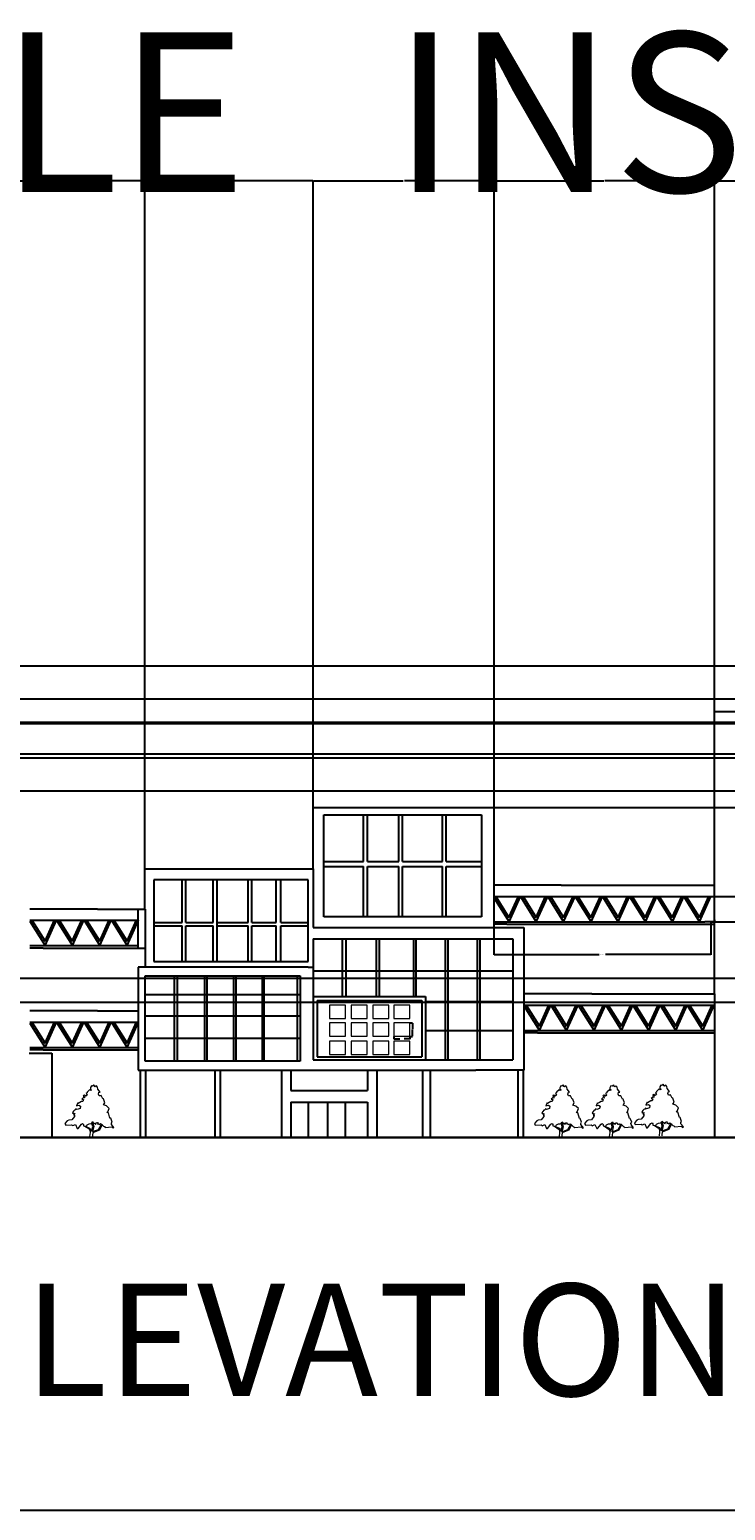
# Model space of a CAD drawing. Units: inches. Extents: x -2248 to 2617, y -128 to 922.
# Tile 3 of 7: x -646 to -152, y -128 to 922. Entities that reach past the tile are written whole.
import ezdxf

# ---------------------------------------------------------------- set-up
doc = ezdxf.new("R2010")
doc.units = ezdxf.units.IN
doc.header["$MEASUREMENT"] = 0
for name, color, linetype, lineweight in [('A-ANNO-DIMS', 2, 'Continuous', 18), ('A-ANNO-TEXT', 7, 'Continuous', 25), ('A-ELEV', 7, 'Continuous', 25), ('A-GLAZ', 4, 'Continuous', 18), ('L-PLNT', 3, 'Continuous', 18)]:
    doc.layers.add(name, color=color, linetype=linetype, lineweight=lineweight)
doc.styles.get("Standard").update_dxf_attribs({"font": 'arial.ttf'})
doc.dimstyles.get("Standard").update_dxf_attribs({"dimtxt": 0.18, "dimasz": 0.18, "dimexe": 0.18, "dimexo": 0.0625, "dimgap": 0.09, "dimtad": 0, "dimtih": 1, "dimtoh": 1, "dimdec": 4, "dimzin": 0, "dimdsep": 46, "dimtxsty": 'Standard', "dimcen": 0.09, "dimadec": 0, "dimazin": 0, "dimtfac": 1, "dimtdec": 4, "dimtofl": 0, "dimtmove": 0, "dimatfit": 3, "dimfxl": 1, "dimtolj": 1, "dimtzin": 0, "dimarcsym": 0})

# ---------------------------------------------------------------- blocks, each defined once
blk = doc.blocks.new('*U2')
for points in [[(22.0124, 137.721), (18.5475, 141.5624), (15.5282, 138.2446), (13.8028, 139.3505), (13.3714, 142.1153), (11.2148, 143.2214), (8.1954, 140.4564), (4.7447, 141.0094), (2.1567, 136.0326), (2.1567, 131.6088), (5.6074, 129.9499), (3.0193, 128.2909), (0.4313, 130.5029), (-6.9015, 123.3141), (-6.9015, 121.6552), (-9.9208, 119.9963), (-9.0581, 118.3373), (-6.9015, 115.0195), (-10.7835, 112.2546), (-14.6656, 115.0195), (-16.8222, 114.4665), (-17.6849, 112.2546), (-14.6656, 111.7016), (-14.2342, 107.2778), (-17.6065, 107.8307), (-21.5669, 103.9599), (-17.2536, 103.4069), (-18.9789, 97.8771), (-22.8609, 97.3241), (-27.1743, 94.5593), (-32.3504, 91.7944), (-32.7817, 94.0063), (-36.6638, 85.7116), (-29.7624, 87.3705), (-25.449, 84.6056), (-26.743, 77.9699), (-34.507, 75.205), (-37.9578, 77.4169), (-39.2518, 74.099), (-42.2711, 73.5461), (-44.8592, 70.2282), (-47.8786, 66.3574), (-43.9965, 63.0395), (-41.4085, 64.6985), (-44.3346, 59.8898), (-42.2089, 60.1377), (-42.5159, 55.7849), (-49.6039, 46.4502), (-58.2307, 45.8972), (-62.1127, 43.6853), (-68.5828, 36.4966), (-65.9947, 32.0727), (-50.0352, 32.6257), (-47.0159, 30.4138), (-39.6831, 33.7317), (-34.507, 22.6721), (-32.3504, 22.6721), (-22.4296, 34.8376), (-19.4102, 36.4966), (-17.2536, 33.7317), (-17.2536, 29.8608), (-13.8028, 28.7549), (-9.0581, 28.7549), (-7.3328, 32.6257), (-1.7254, 35.3906), (3.8821, 35.9436), (6.4701, 38.1555), (6.9014, 38.7085), (8.1954, 41.4734), (9.9208, 40.3674), (11.2148, 35.9436), (14.2341, 37.6025), (15.0968, 36.4966), (15.9595, 33.7317), (18.9789, 38.7085), (21.9982, 38.7085), (23.2922, 36.4966), (21.9982, 34.2847), (25.4489, 35.3906), (26.743, 33.7317), (29.7623, 35.9436), (32.7817, 34.8376), (38.8204, 28.7549), (41.4084, 27.6489), (43.5651, 25.437), (61.6813, 27.0959), (65.132, 23.7781), (67.7201, 24.884), (60.8186, 33.7317), (60.3873, 37.0495), (62.544, 40.3674), (58.662, 50.874), (56.5053, 50.874), (52.1919, 66.3574), (47.8785, 66.9103), (50.4665, 69.1222), (53.9172, 77.9699), (47.0158, 85.1586), (38.3891, 87.9235), (42.2711, 94.0063)], [(42.2711, 94.0063), (38.8204, 104.5129), (36.6637, 104.5129), (32.3503, 113.9135), (29.7623, 113.3605), (26.743, 113.3605), (24.5862, 117.7844), (25.8802, 123.8671), (29.331, 123.8671), (22.8609, 131.6088), (21.9982, 137.6916)], [(-12.9401, 28.7549), (-2.588, 22.1191), (0.8626, 17.6953), (1.7253, 11.6125), (0, 0)], [(-9.9208, 28.2019), (0, 23.2251), (3.4507, 19.9072), (4.7447, 15.4834), (8.6267, 27.0959), (6.4701, 37.6025)], [(34.5071, 33.1787), (27.1743, 18.2483), (9.0581, 10.5066), (7.7641, 3.8708), (8.1954, 0)], [(8.1954, 40.3674), (11.2148, 27.6489), (8.1954, 13.8245), (24.5862, 19.9072), (32.7817, 34.2847)]]:
    blk.add_lwpolyline(points)
blk = doc.blocks.new('TRUSS-BRIDGE-SEG')
for p, q in [((0, 17.2), (10.8, 0)), ((10.8, 0), (18.9, 17.9)), ((18.8, 17.9), (30.1, 0)), ((30.1, 0), (38.2, 17.9)), ((38.3, 17.9), (49.5, 0)), ((49.5, 0), (57.6, 17.9)), ((57.7, 17.9), (69, 0)), ((69, 0), (77.1, 17.9)), ((77, 17.9), (88.2, 0)), ((88.2, 0), (96.3, 17.9)), ((96.3, 17.9), (107.5, 0)), ((107.5, 0), (115.6, 17.9)), ((115.5, 17.9), (126.7, 0)), ((126.7, 0), (134.8, 17.9)), ((134.7, 17.9), (145.9, 0)), ((145.9, 0), (154, 17.9))]:
    blk.add_line(p, q)
blk = doc.blocks.new('WIN-SMALL')
for p, q in [((0, 9.6), (0, 0)), ((11.4, 9.6), (0, 9.6)), ((0, 0), (11.4, 0)), ((11.4, 0), (11.4, 9.6))]:
    blk.add_line(p, q)
blk = doc.blocks.new('*D8')
at = {"layer": 'A-ANNO-DIMS', "color": 0, "lineweight": -2, "transparency": 16777216}
for p, q in [((-387.2, 208.1), (-387.2, 206.2)), ((-387, 206.4), (-383.1, 206.4)), ((-376, 206.4), (-380, 206.4)), ((-375.8, 208.1), (-375.8, 206.2))]:
    blk.add_line(p, q, dxfattribs=at)
at = {"layer": 'A-ANNO-DIMS', "color": 0, "transparency": 16777216}
for points in [[(-387, 206.5), (-387, 206.4), (-387.2, 206.4)], [(-376, 206.5), (-376, 206.4), (-375.8, 206.4)]]:
    blk.add_solid(points, dxfattribs=at)
at = {"layer": 'Defpoints', "color": 0, "transparency": 16777216}
for p in [(-387.2, 208.1), (-375.8, 208.1), (-375.8, 206.4)]:
    blk.add_point(p, dxfattribs=at)
at = {"layer": 'A-ANNO-DIMS', "color": 0, "transparency": 16777216, "insert": (-381.5, 206.4), "char_height": 0.18, "attachment_point": 5}
blk.add_mtext('\\A1;SMALL WINDOW 11 TYP.', dxfattribs=at)
blk = doc.blocks.new('*D9')
at = {"layer": 'A-ANNO-DIMS', "color": 0, "lineweight": -2, "transparency": 16777216}
for p, q in [((-375.8, 217.7), (-374, 217.7)), ((-374.1, 217.5), (-374.1, 213.1)), ((-374.1, 208.3), (-374.1, 212.7)), ((-375.8, 208.1), (-374, 208.1))]:
    blk.add_line(p, q, dxfattribs=at)
at = {"layer": 'A-ANNO-DIMS', "color": 0, "transparency": 16777216}
for points in [[(-374.2, 217.5), (-374.1, 217.5), (-374.1, 217.7)], [(-374.2, 208.3), (-374.1, 208.3), (-374.1, 208.1)]]:
    blk.add_solid(points, dxfattribs=at)
at = {"layer": 'Defpoints', "color": 0, "transparency": 16777216}
for p in [(-375.8, 217.7), (-374.1, 217.7), (-375.8, 208.1)]:
    blk.add_point(p, dxfattribs=at)
at = {"layer": 'A-ANNO-DIMS', "color": 0, "transparency": 16777216, "insert": (-374.1, 212.9), "char_height": 0.18, "attachment_point": 5}
blk.add_mtext('\\A1;10 TYP.', dxfattribs=at)
blk = doc.blocks.new('*D14')
at = {"layer": 'A-ANNO-DIMS', "color": 0, "lineweight": -2, "transparency": 16777216}
for p, q in [((-316.3, 289.2), (-316.3, 266)), ((-162.4, 289.2), (-162.4, 266)), ((-316.1, 266.2), (-241.6, 266.2)), ((-162.5, 266.2), (-237.1, 266.2))]:
    blk.add_line(p, q, dxfattribs=at)
at = {"layer": 'A-ANNO-DIMS', "color": 0, "transparency": 16777216}
for points in [[(-316.1, 266.2), (-316.1, 266.2), (-316.3, 266.2)], [(-162.5, 266.2), (-162.5, 266.2), (-162.4, 266.2)]]:
    blk.add_solid(points, dxfattribs=at)
at = {"layer": 'Defpoints', "color": 0, "transparency": 16777216}
for p in [(-316.3, 289.3), (-162.4, 289.3), (-162.4, 266.2)]:
    blk.add_point(p, dxfattribs=at)
at = {"layer": 'A-ANNO-DIMS', "color": 0, "transparency": 16777216, "insert": (-239.3, 266.2), "char_height": 0.18, "attachment_point": 5}
blk.add_mtext('\\A1;TRUSS BRIDGE SEGMENT 154 TYP.', dxfattribs=at)
blk = doc.blocks.new('*D15')
at = {"layer": 'A-ANNO-DIMS', "color": 0, "lineweight": -2, "transparency": 16777216}
for p, q in [((-162.3, 307.2), (-139.1, 307.2)), ((-139.3, 307), (-139.3, 298.4)), ((-139.3, 289.5), (-139.3, 298.1)), ((-162.3, 289.3), (-139.1, 289.3))]:
    blk.add_line(p, q, dxfattribs=at)
at = {"layer": 'A-ANNO-DIMS', "color": 0, "transparency": 16777216}
for points in [[(-139.3, 307), (-139.2, 307), (-139.3, 307.2)], [(-139.3, 289.5), (-139.2, 289.5), (-139.3, 289.3)]]:
    blk.add_solid(points, dxfattribs=at)
at = {"layer": 'Defpoints', "color": 0, "transparency": 16777216}
for p in [(-162.4, 307.2), (-139.3, 307.2), (-162.4, 289.3)]:
    blk.add_point(p, dxfattribs=at)
at = {"layer": 'A-ANNO-DIMS', "color": 0, "transparency": 16777216, "insert": (-139.3, 298.2), "char_height": 0.18, "attachment_point": 5}
blk.add_mtext('\\A1;18 TYP.', dxfattribs=at)
blk = doc.blocks.new('*D20')
at = {"layer": 'A-ANNO-DIMS', "color": 0, "lineweight": -2, "transparency": 16777216}
for p, q in [((-1595.3, 429.9), (2616.5, 429.9)), ((2616.3, 429.7), (2616.3, 417.9)), ((2616.3, 405.8), (2616.3, 417.5)), ((-1653.9, 405.6), (2616.5, 405.6))]:
    blk.add_line(p, q, dxfattribs=at)
at = {"layer": 'A-ANNO-DIMS', "color": 0, "transparency": 16777216}
for points in [[(2616.2, 429.7), (2616.3, 429.7), (2616.3, 429.9)], [(2616.2, 405.8), (2616.3, 405.8), (2616.3, 405.6)]]:
    blk.add_solid(points, dxfattribs=at)
at = {"layer": 'Defpoints', "color": 0, "transparency": 16777216}
for p in [(-1595.4, 429.9), (-1654, 405.6), (2616.3, 405.6)]:
    blk.add_point(p, dxfattribs=at)
at = {"layer": 'A-ANNO-DIMS', "color": 0, "transparency": 16777216, "insert": (2616.3, 417.7), "char_height": 0.18, "attachment_point": 5}
blk.add_mtext('\\A1;24.3', dxfattribs=at)
blk = doc.blocks.new('*D21')
at = {"layer": 'A-ANNO-DIMS', "color": 0, "lineweight": -2, "transparency": 16777216}
for p, q in [((-1125.3, 470.6), (2616.5, 470.6)), ((2616.3, 470.4), (2616.3, 451)), ((2616.3, 431.1), (2616.3, 450.6)), ((-1257.9, 430.9), (2616.5, 430.9))]:
    blk.add_line(p, q, dxfattribs=at)
at = {"layer": 'A-ANNO-DIMS', "color": 0, "transparency": 16777216}
for points in [[(2616.2, 470.4), (2616.3, 470.4), (2616.3, 470.6)], [(2616.2, 431.1), (2616.3, 431.1), (2616.3, 430.9)]]:
    blk.add_solid(points, dxfattribs=at)
at = {"layer": 'Defpoints', "color": 0, "transparency": 16777216}
for p in [(-1125.4, 470.6), (-1258, 430.9), (2616.3, 430.9)]:
    blk.add_point(p, dxfattribs=at)
at = {"layer": 'A-ANNO-DIMS', "color": 0, "transparency": 16777216, "insert": (2616.3, 450.8), "char_height": 0.18, "attachment_point": 5}
blk.add_mtext('\\A1;39.705', dxfattribs=at)
blk = doc.blocks.new('*D22')
at = {"layer": 'A-ANNO-DIMS', "color": 0, "lineweight": -2, "transparency": 16777216}
for p, q in [((-733.3, 408.4), (2616.5, 408.4)), ((2616.3, 408.2), (2616.3, 329.1)), ((2616.3, 249.6), (2616.3, 328.7)), ((-719.1, 249.4), (2616.5, 249.4))]:
    blk.add_line(p, q, dxfattribs=at)
at = {"layer": 'A-ANNO-DIMS', "color": 0, "transparency": 16777216}
for points in [[(2616.2, 408.2), (2616.3, 408.2), (2616.3, 408.4)], [(2616.2, 249.6), (2616.3, 249.6), (2616.3, 249.4)]]:
    blk.add_solid(points, dxfattribs=at)
at = {"layer": 'Defpoints', "color": 0, "transparency": 16777216}
for p in [(-733.4, 408.4), (-719.2, 249.4), (2616.3, 249.4)]:
    blk.add_point(p, dxfattribs=at)
at = {"layer": 'A-ANNO-DIMS', "color": 0, "transparency": 16777216, "insert": (2616.3, 328.9), "char_height": 0.18, "attachment_point": 5}
blk.add_mtext('\\A1;159.02', dxfattribs=at)
blk = doc.blocks.new('*D23')
at = {"layer": 'A-ANNO-DIMS', "color": 0, "lineweight": -2, "transparency": 16777216}
for p, q in [((-719.1, 249.4), (2616.5, 249.4)), ((2616.3, 249.2), (2616.3, 193.1)), ((2616.3, 136.6), (2616.3, 192.7)), ((-719.1, 136.5), (2616.5, 136.5))]:
    blk.add_line(p, q, dxfattribs=at)
at = {"layer": 'A-ANNO-DIMS', "color": 0, "transparency": 16777216}
for points in [[(2616.2, 249.2), (2616.3, 249.2), (2616.3, 249.4)], [(2616.2, 136.6), (2616.3, 136.6), (2616.3, 136.5)]]:
    blk.add_solid(points, dxfattribs=at)
at = {"layer": 'Defpoints', "color": 0, "transparency": 16777216}
for p in [(-719.2, 249.4), (-719.2, 136.5), (2616.3, 136.5)]:
    blk.add_point(p, dxfattribs=at)
at = {"layer": 'A-ANNO-DIMS', "color": 0, "transparency": 16777216, "insert": (2616.3, 192.9), "char_height": 0.18, "attachment_point": 5}
blk.add_mtext('\\A1;112.94', dxfattribs=at)
blk = doc.blocks.new('*D24')
at = {"layer": 'A-ANNO-DIMS', "color": 0, "lineweight": -2, "transparency": 16777216}
for p, q in [((-316.1, 370.3), (2616.5, 370.3)), ((2616.3, 370.1), (2616.3, 253.6)), ((2616.3, 136.6), (2616.3, 253.2)), ((-159.8, 136.5), (2616.5, 136.5))]:
    blk.add_line(p, q, dxfattribs=at)
at = {"layer": 'A-ANNO-DIMS', "color": 0, "transparency": 16777216}
for points in [[(2616.2, 370.1), (2616.3, 370.1), (2616.3, 370.3)], [(2616.2, 136.6), (2616.3, 136.6), (2616.3, 136.5)]]:
    blk.add_solid(points, dxfattribs=at)
at = {"layer": 'Defpoints', "color": 0, "transparency": 16777216}
for p in [(-316.2, 370.3), (-159.9, 136.5), (2616.3, 136.5)]:
    blk.add_point(p, dxfattribs=at)
at = {"layer": 'A-ANNO-DIMS', "color": 0, "transparency": 16777216, "insert": (2616.3, 253.4), "char_height": 0.18, "attachment_point": 5}
blk.add_mtext('\\A1;233.87', dxfattribs=at)
blk = doc.blocks.new('*D29')
at = {"layer": 'A-ANNO-DIMS', "color": 0, "lineweight": -2, "transparency": 16777216}
for p, q in [((358.9, 382), (-2247.7, 382)), ((-2247.5, 381.8), (-2247.5, 259.4)), ((-2247.5, 136.6), (-2247.5, 259)), ((392.6, 136.5), (-2247.7, 136.5))]:
    blk.add_line(p, q, dxfattribs=at)
at = {"layer": 'A-ANNO-DIMS', "color": 0, "transparency": 16777216}
for points in [[(-2247.5, 381.8), (-2247.5, 381.8), (-2247.5, 382)], [(-2247.5, 136.6), (-2247.5, 136.6), (-2247.5, 136.5)]]:
    blk.add_solid(points, dxfattribs=at)
at = {"layer": 'Defpoints', "color": 0, "transparency": 16777216}
for p in [(359, 382), (-2247.5, 136.5), (392.7, 136.5)]:
    blk.add_point(p, dxfattribs=at)
at = {"layer": 'A-ANNO-DIMS', "color": 0, "transparency": 16777216, "insert": (-2247.5, 259.2), "char_height": 0.18, "attachment_point": 5}
blk.add_mtext('\\A1;245.5', dxfattribs=at)
blk = doc.blocks.new('*D30')
at = {"layer": 'A-ANNO-DIMS', "color": 0, "lineweight": -2, "transparency": 16777216}
for p, q in [((201.8, 232.1), (-2247.7, 232.1)), ((-2247.5, 231.9), (-2247.5, 184.4)), ((-2247.5, 136.6), (-2247.5, 184.1)), ((210.7, 136.5), (-2247.7, 136.5))]:
    blk.add_line(p, q, dxfattribs=at)
at = {"layer": 'A-ANNO-DIMS', "color": 0, "transparency": 16777216}
for points in [[(-2247.5, 231.9), (-2247.5, 231.9), (-2247.5, 232.1)], [(-2247.5, 136.6), (-2247.5, 136.6), (-2247.5, 136.5)]]:
    blk.add_solid(points, dxfattribs=at)
at = {"layer": 'Defpoints', "color": 0, "transparency": 16777216}
for p in [(201.8, 232.1), (-2247.5, 136.5), (210.8, 136.5)]:
    blk.add_point(p, dxfattribs=at)
at = {"layer": 'A-ANNO-DIMS', "color": 0, "transparency": 16777216, "insert": (-2247.5, 184.3), "char_height": 0.18, "attachment_point": 5}
blk.add_mtext('\\A1;95.6', dxfattribs=at)
blk = doc.blocks.new('*D31')
at = {"layer": 'A-ANNO-DIMS', "color": 0, "lineweight": -2, "transparency": 16777216}
for p, q in [((934.8, 447.2), (-2247.7, 447.2)), ((-2247.5, 447), (-2247.5, 292)), ((-2247.5, 136.6), (-2247.5, 291.6)), ((820, 136.5), (-2247.7, 136.5))]:
    blk.add_line(p, q, dxfattribs=at)
at = {"layer": 'A-ANNO-DIMS', "color": 0, "transparency": 16777216}
for points in [[(-2247.5, 447), (-2247.5, 447), (-2247.5, 447.2)], [(-2247.5, 136.6), (-2247.5, 136.6), (-2247.5, 136.5)]]:
    blk.add_solid(points, dxfattribs=at)
at = {"layer": 'Defpoints', "color": 0, "transparency": 16777216}
for p in [(934.9, 447.2), (-2247.5, 136.5), (820.1, 136.5)]:
    blk.add_point(p, dxfattribs=at)
at = {"layer": 'A-ANNO-DIMS', "color": 0, "transparency": 16777216, "insert": (-2247.5, 291.8), "char_height": 0.18, "attachment_point": 5}
blk.add_mtext('\\A1;310.7', dxfattribs=at)
blk = doc.blocks.new('*D33')
at = {"layer": 'A-ANNO-DIMS', "color": 0, "lineweight": -2, "transparency": 16777216}
for p, q in [((2393, 136.4), (2393, -127.9)), ((-2024.3, 122), (-2024.3, -127.9)), ((-2024.1, -127.7), (184, -127.7)), ((2392.8, -127.7), (184.7, -127.7))]:
    blk.add_line(p, q, dxfattribs=at)
at = {"layer": 'A-ANNO-DIMS', "color": 0, "transparency": 16777216}
for points in [[(-2024.1, -127.6), (-2024.1, -127.7), (-2024.3, -127.7)], [(2392.8, -127.6), (2392.8, -127.7), (2393, -127.7)]]:
    blk.add_solid(points, dxfattribs=at)
at = {"layer": 'Defpoints', "color": 0, "transparency": 16777216}
for p in [(2393, 136.5), (-2024.3, 122.1), (2393, -127.7)]:
    blk.add_point(p, dxfattribs=at)
at = {"layer": 'A-ANNO-DIMS', "color": 0, "transparency": 16777216, "insert": (184.4, -127.7), "char_height": 0.18, "attachment_point": 5}
blk.add_mtext('\\A1;4417', dxfattribs=at)
blk = doc.blocks.new('*D41')
at = {"layer": 'A-ANNO-DIMS', "color": 0, "lineweight": -2, "transparency": 16777216}
for p, q in [((-733.4, 408.5), (-733.4, 814.7)), ((-733.2, 814.5), (-649, 814.5)), ((-564.1, 814.5), (-648.2, 814.5)), ((-563.9, 327), (-563.9, 814.7))]:
    blk.add_line(p, q, dxfattribs=at)
at = {"layer": 'A-ANNO-DIMS', "color": 0, "transparency": 16777216}
for points in [[(-733.2, 814.5), (-733.2, 814.5), (-733.4, 814.5)], [(-564.1, 814.5), (-564.1, 814.5), (-563.9, 814.5)]]:
    blk.add_solid(points, dxfattribs=at)
at = {"layer": 'Defpoints', "color": 0, "transparency": 16777216}
for p in [(-563.9, 814.5), (-733.4, 408.4), (-563.9, 326.9)]:
    blk.add_point(p, dxfattribs=at)
at = {"layer": 'A-ANNO-DIMS', "color": 0, "transparency": 16777216, "insert": (-648.6, 814.5), "char_height": 0.18, "attachment_point": 5}
blk.add_mtext('\\A1;169.5', dxfattribs=at)
blk = doc.blocks.new('*D42')
at = {"layer": 'A-ANNO-DIMS', "color": 0, "lineweight": -2, "transparency": 16777216}
for p, q in [((-563.9, 327), (-563.9, 814.7)), ((-563.7, 814.5), (-504.5, 814.5)), ((-444.6, 814.5), (-503.7, 814.5)), ((-444.4, 327), (-444.4, 814.7))]:
    blk.add_line(p, q, dxfattribs=at)
at = {"layer": 'A-ANNO-DIMS', "color": 0, "transparency": 16777216}
for points in [[(-563.7, 814.5), (-563.7, 814.5), (-563.9, 814.5)], [(-444.6, 814.5), (-444.6, 814.5), (-444.4, 814.5)]]:
    blk.add_solid(points, dxfattribs=at)
at = {"layer": 'Defpoints', "color": 0, "transparency": 16777216}
for p in [(-444.4, 814.5), (-563.9, 326.9), (-444.4, 326.9)]:
    blk.add_point(p, dxfattribs=at)
at = {"layer": 'A-ANNO-DIMS', "color": 0, "transparency": 16777216, "insert": (-504.1, 814.5), "char_height": 0.18, "attachment_point": 5}
blk.add_mtext('\\A1;119.5', dxfattribs=at)
blk = doc.blocks.new('*D43')
at = {"layer": 'A-ANNO-DIMS', "color": 0, "lineweight": -2, "transparency": 16777216}
for p, q in [((-444.4, 370.4), (-444.4, 814.7)), ((-444.2, 814.5), (-380.7, 814.5)), ((-316.4, 814.5), (-379.8, 814.5)), ((-316.2, 370.4), (-316.2, 814.7))]:
    blk.add_line(p, q, dxfattribs=at)
at = {"layer": 'A-ANNO-DIMS', "color": 0, "transparency": 16777216}
for points in [[(-444.2, 814.5), (-444.2, 814.5), (-444.4, 814.5)], [(-316.4, 814.5), (-316.4, 814.5), (-316.2, 814.5)]]:
    blk.add_solid(points, dxfattribs=at)
at = {"layer": 'Defpoints', "color": 0, "transparency": 16777216}
for p in [(-316.2, 814.5), (-444.4, 370.3), (-316.2, 370.3)]:
    blk.add_point(p, dxfattribs=at)
at = {"layer": 'A-ANNO-DIMS', "color": 0, "transparency": 16777216, "insert": (-380.3, 814.5), "char_height": 0.18, "attachment_point": 5}
blk.add_mtext('\\A1;128.17', dxfattribs=at)
blk = doc.blocks.new('*D44')
at = {"layer": 'A-ANNO-DIMS', "color": 0, "lineweight": -2, "transparency": 16777216}
for p, q in [((-316.2, 370.4), (-316.2, 814.7)), ((-316, 814.5), (-238.4, 814.5)), ((-160.1, 814.5), (-237.7, 814.5)), ((-159.9, 438.5), (-159.9, 814.7))]:
    blk.add_line(p, q, dxfattribs=at)
at = {"layer": 'A-ANNO-DIMS', "color": 0, "transparency": 16777216}
for points in [[(-316, 814.5), (-316, 814.5), (-316.2, 814.5)], [(-160.1, 814.5), (-160.1, 814.5), (-159.9, 814.5)]]:
    blk.add_solid(points, dxfattribs=at)
at = {"layer": 'Defpoints', "color": 0, "transparency": 16777216}
for p in [(-159.9, 814.5), (-159.9, 438.4), (-316.2, 370.3)]:
    blk.add_point(p, dxfattribs=at)
at = {"layer": 'A-ANNO-DIMS', "color": 0, "transparency": 16777216, "insert": (-238.1, 814.5), "char_height": 0.18, "attachment_point": 5}
blk.add_mtext('\\A1;156.3', dxfattribs=at)
blk = doc.blocks.new('*D45')
at = {"layer": 'A-ANNO-DIMS', "color": 0, "lineweight": -2, "transparency": 16777216}
for p, q in [((-159.9, 438.5), (-159.9, 814.7)), ((-159.7, 814.5), (-57.5, 814.5)), ((45.6, 814.5), (-56.6, 814.5)), ((45.8, 438.5), (45.8, 814.7))]:
    blk.add_line(p, q, dxfattribs=at)
at = {"layer": 'A-ANNO-DIMS', "color": 0, "transparency": 16777216}
for points in [[(-159.7, 814.5), (-159.7, 814.5), (-159.9, 814.5)], [(45.6, 814.5), (45.6, 814.5), (45.8, 814.5)]]:
    blk.add_solid(points, dxfattribs=at)
at = {"layer": 'Defpoints', "color": 0, "transparency": 16777216}
for p in [(45.8, 814.5), (-159.9, 438.4), (45.8, 438.4)]:
    blk.add_point(p, dxfattribs=at)
at = {"layer": 'A-ANNO-DIMS', "color": 0, "transparency": 16777216, "insert": (-57, 814.5), "char_height": 0.18, "attachment_point": 5}
blk.add_mtext('\\A1;205.73', dxfattribs=at)

msp = doc.modelspace()

# ---------------------------------------------------------------- linework, layer by layer
at = {"layer": 'A-ELEV'}
for p, q in [((-159.9067, 399.7951), (-159.9067, 438.443)), ((-159.9067, 438.443), (3.2456, 438.443)), ((-159.9067, 351.7702), (-159.9067, 399.7951)), ((-444.3761, 326.8999), (-444.3761, 370.3211)), ((-444.3761, 370.3211), (-316.2025, 370.3211)), ((-316.2025, 370.3211), (-316.2025, 285.327)), ((-436.7944, 292.802), (-436.7944, 365.1857)), ((-436.7944, 365.1857), (-325.0903, 365.1857)), ((-408.8752, 332.0264), (-408.8752, 365.1857)), ((-405.9836, 332.0264), (-405.9836, 365.1857)), ((-383.6774, 332.0264), (-383.6774, 365.1857)), ((-380.9924, 332.0264), (-380.9924, 365.1857)), ((-352.6966, 332.0264), (-352.6966, 365.1857)), ((-350.0116, 332.0264), (-350.0116, 365.1857)), ((-325.0903, 365.1857), (-325.0903, 292.802)), ((-159.9067, 268.3497), (-159.9067, 351.7702)), ((-563.8805, 298.3514), (-563.8805, 326.8999)), ((-563.8805, 326.8999), (-444.3761, 326.8999)), ((-444.3761, 326.8999), (-444.3761, 285.327)), ((-436.7944, 332.0264), (-408.8752, 332.0264)), ((-436.7944, 328.4956), (-408.8752, 328.4956)), ((-408.8752, 292.802), (-408.8752, 328.4956)), ((-405.9836, 332.0264), (-383.6774, 332.0264)), ((-405.9836, 292.802), (-405.9836, 328.4956)), ((-405.9836, 328.4956), (-383.6774, 328.4956)), ((-383.6774, 292.802), (-383.6774, 328.4956)), ((-380.9924, 332.0264), (-352.6966, 332.0264)), ((-380.9924, 292.802), (-380.9924, 328.4956)), ((-380.9924, 328.4956), (-352.6966, 328.4956)), ((-352.6966, 292.802), (-352.6966, 328.4956)), ((-350.0116, 332.0264), (-325.0903, 332.0264)), ((-350.0116, 292.802), (-350.0116, 328.4956)), ((-350.0116, 328.4956), (-325.0903, 328.4956)), ((-557.424, 319.0965), (-557.424, 298.3514)), ((-447.9914, 319.0965), (-557.424, 319.0965)), ((-537.4402, 288.7204), (-537.4402, 319.0965)), ((-534.7695, 288.7204), (-534.7695, 319.0965)), ((-515.3335, 288.7204), (-515.3335, 319.0965)), ((-512.4402, 261.2094), (-512.4402, 319.0965)), ((-490.5471, 288.7204), (-490.5471, 319.0965)), ((-487.9584, 288.7204), (-487.9584, 319.0965)), ((-470.785, 288.7204), (-470.785, 319.0965)), ((-467.4827, 288.7204), (-467.4827, 319.0965)), ((-447.9914, 261.2094), (-447.9914, 319.0965)), ((-268.5067, 315.183), (-316.3159, 315.183)), ((-268.5067, 315.183), (-159.9067, 315.183)), ((-163.4279, 315.183), (-159.9067, 315.183)), ((-159.9067, 290.7409), (-159.9067, 315.183)), ((-316.3159, 307.2132), (-159.9067, 307.2132)), ((-314.9029, 307.2075), (-305.6236, 292.355)), ((-305.6236, 292.355), (-298.911, 307.2132)), ((-295.6263, 307.2075), (-286.3469, 292.355)), ((-286.3469, 292.355), (-279.6343, 307.2132)), ((-276.1493, 307.2075), (-266.87, 292.355)), ((-266.87, 292.355), (-260.1574, 307.2132)), ((-256.7297, 307.2075), (-247.4503, 292.355)), ((-247.4503, 292.355), (-240.7377, 307.2132)), ((-237.4427, 307.2075), (-228.1634, 292.355)), ((-228.1634, 292.355), (-221.4508, 307.2132)), ((-218.1558, 307.2075), (-208.8765, 292.355)), ((-208.8765, 292.355), (-202.1639, 307.2132)), ((-199.0162, 307.2075), (-189.7368, 292.355)), ((-189.7368, 292.355), (-183.0243, 307.2132)), ((-179.8243, 307.2075), (-170.5449, 292.355)), ((-170.5449, 292.355), (-163.8323, 307.2132)), ((-597.5248, 298.3514), (-645.3339, 298.3514)), ((-597.5248, 298.3514), (-568.2898, 298.3514)), ((-568.6968, 290.3816), (-568.6968, 298.3514)), ((-568.6968, 298.3514), (-563.8805, 298.3514)), ((-563.5285, 298.3514), (-563.5285, 261.2094)), ((-557.424, 298.3514), (-557.424, 261.2094)), ((-645.3339, 290.3816), (-568.2898, 290.3816)), ((-645.3339, 289.6982), (-634.5569, 272.4486)), ((-643.921, 290.3759), (-634.6416, 275.5235)), ((-634.6416, 275.5235), (-627.929, 290.3816)), ((-634.5569, 272.4486), (-626.4558, 290.3802)), ((-626.4843, 290.3816), (-615.2803, 272.4486)), ((-624.6443, 290.3759), (-615.365, 275.5235)), ((-615.365, 275.5235), (-608.6524, 290.3816)), ((-615.2803, 272.4486), (-607.1792, 290.3802)), ((-607.0073, 290.3816), (-595.8033, 272.4486)), ((-605.1674, 290.3759), (-595.888, 275.5235)), ((-595.888, 275.5235), (-589.1754, 290.3816)), ((-595.8033, 272.4486), (-587.7022, 290.3802)), ((-587.5877, 290.3816), (-576.3837, 272.4486)), ((-585.7477, 290.3759), (-576.4684, 275.5235)), ((-576.4684, 275.5235), (-569.7558, 290.3816)), ((-576.3837, 272.4486), (-568.2826, 290.3802)), ((-568.6968, 270.6767), (-568.6968, 290.3816)), ((-568.3008, 290.3816), (-568.2898, 290.3641)), ((-557.424, 288.7204), (-537.4402, 288.7204)), ((-557.424, 286.4974), (-537.4402, 286.4974)), ((-537.4402, 261.2094), (-537.4402, 286.4974)), ((-534.7695, 288.7204), (-515.3335, 288.7204)), ((-534.7695, 261.2094), (-534.7695, 286.4974)), ((-534.7695, 286.4974), (-515.3335, 286.4974)), ((-515.3335, 261.2094), (-515.3335, 286.4974)), ((-512.4402, 288.7204), (-490.5471, 288.7204)), ((-512.4402, 286.4974), (-490.5471, 286.4974)), ((-490.5471, 261.2094), (-490.5471, 286.4974)), ((-487.9584, 288.7204), (-470.785, 288.7204)), ((-487.9584, 261.2094), (-487.9584, 286.4974)), ((-487.9584, 286.4974), (-470.785, 286.4974)), ((-470.785, 261.2094), (-470.785, 286.4974)), ((-467.4827, 288.7204), (-447.9914, 288.7204)), ((-467.4827, 261.2094), (-467.4827, 286.4974)), ((-467.4827, 286.4974), (-447.9914, 286.4974)), ((-444.3761, 285.327), (-295.0449, 285.327)), ((-325.0903, 292.802), (-436.7944, 292.802)), ((-316.3159, 289.2624), (-168.2441, 289.2624)), ((-307.011, 287.5083), (-316.3159, 287.5083)), ((-307.011, 287.5083), (-179.9927, 287.5083)), ((-295.0449, 285.327), (-295.0449, 184.1492)), ((-211.2213, 289.2624), (-211.2064, 289.2297)), ((-211.2064, 289.2297), (-211.1885, 289.2624)), ((-179.9927, 287.5083), (-168.2441, 287.5083)), ((-168.2441, 289.2624), (-166.5893, 289.2624)), ((-168.2441, 287.5083), (-159.9067, 287.5083)), ((-159.9067, 289.2624), (-166.5893, 289.2624)), ((-159.9067, 290.7409), (-159.9067, 289.2624)), ((-444.3761, 277.2905), (-302.8706, 277.2905)), ((-444.3761, 277.2905), (-444.3761, 257.0722)), ((-423.8025, 277.2905), (-423.8025, 236.274)), ((-421.253, 277.2905), (-421.253, 236.274)), ((-399.8375, 277.2905), (-399.8375, 236.274)), ((-397.543, 277.2905), (-397.543, 236.274)), ((-373.323, 277.2905), (-373.323, 236.274)), ((-371.5384, 277.2905), (-371.5384, 236.274)), ((-350.8877, 277.2905), (-350.8877, 191.5165)), ((-348.8481, 277.2905), (-348.8481, 191.5165)), ((-328.1974, 277.2905), (-328.1974, 191.5165)), ((-326.1579, 277.2905), (-326.1579, 191.5165)), ((-302.8706, 277.2905), (-302.8706, 191.5165)), ((-645.3339, 272.4308), (-568.2898, 272.4308)), ((-636.029, 270.6767), (-645.3339, 270.6767)), ((-636.029, 270.6767), (-568.2898, 270.6767)), ((-568.6968, 270.6767), (-563.5285, 270.6767)), ((-159.9067, 238.2214), (-159.9067, 268.3497)), ((-568.6968, 257.0722), (-568.6968, 184.1492)), ((-447.9914, 257.0722), (-568.6968, 257.0722)), ((-563.5285, 261.2094), (-563.5371, 257.0722)), ((-557.424, 261.2094), (-447.9914, 261.2094)), ((-447.9914, 257.0722), (-444.3761, 257.0722)), ((-444.3761, 257.0722), (-444.3761, 191.5165)), ((-444.3761, 254.5663), (-302.8706, 254.5663)), ((-563.5496, 251.0795), (-453.6192, 251.0795)), ((-563.5496, 190.6029), (-563.5496, 251.0795)), ((-542.8027, 190.6029), (-542.8027, 251.0795)), ((-540.6499, 190.6029), (-540.6499, 251.0795)), ((-521.2921, 190.6029), (-521.2921, 251.0795)), ((-519.6216, 190.6029), (-519.6216, 251.0795)), ((-500.8313, 190.6029), (-500.8313, 251.0795)), ((-499.1609, 190.6029), (-499.1609, 251.0795)), ((-480.3926, 190.6029), (-480.3926, 251.0795)), ((-479.2135, 190.6029), (-479.2135, 251.0795)), ((-455.6303, 190.6029), (-455.6303, 251.0795)), ((-453.6192, 251.0795), (-453.6192, 190.6029)), ((-563.5496, 237.7951), (-453.6192, 237.7951)), ((-444.3761, 236.274), (-364.6935, 236.274)), ((-441.7224, 233.5562), (-367.38, 233.5562)), ((-441.7224, 233.5562), (-441.7224, 193.6443)), ((-367.38, 233.5562), (-367.38, 193.6443)), ((-364.6935, 236.274), (-364.6935, 191.5165)), ((-364.6935, 232.7064), (-302.8706, 232.7064)), ((-246.9086, 238.2214), (-294.7178, 238.2214)), ((-246.9086, 238.2214), (-159.9067, 238.2214)), ((-159.9067, 238.2214), (-159.9067, 210.5467)), ((-597.5248, 226.2211), (-645.3339, 226.2211)), ((-597.5248, 226.2211), (-568.2898, 226.2211)), ((-563.5496, 222.5863), (-453.6192, 222.5863)), ((-294.7178, 230.2515), (-159.9067, 230.2515)), ((-294.7178, 229.5681), (-283.9407, 212.3185)), ((-293.3048, 230.2458), (-284.0254, 215.3934)), ((-284.0254, 215.3934), (-277.3128, 230.2515)), ((-283.9407, 212.3185), (-275.8396, 230.2501)), ((-275.8681, 230.2515), (-264.6641, 212.3185)), ((-274.0281, 230.2458), (-264.7488, 215.3934)), ((-264.7488, 215.3934), (-258.0362, 230.2515)), ((-264.6641, 212.3185), (-256.563, 230.2501)), ((-256.3912, 230.2515), (-245.1871, 212.3185)), ((-254.5512, 230.2458), (-245.2718, 215.3934)), ((-245.2718, 215.3934), (-238.5593, 230.2515)), ((-245.1871, 212.3185), (-237.086, 230.2501)), ((-236.9715, 230.2515), (-225.7675, 212.3185)), ((-235.1315, 230.2458), (-225.8522, 215.3934)), ((-225.8522, 215.3934), (-219.1396, 230.2515)), ((-225.7675, 212.3185), (-217.6664, 230.2501)), ((-217.6846, 230.2515), (-206.4806, 212.3185)), ((-215.8446, 230.2458), (-206.5653, 215.3934)), ((-206.5653, 215.3934), (-199.8527, 230.2515)), ((-206.4806, 212.3185), (-198.3795, 230.2501)), ((-198.3977, 230.2515), (-187.1937, 212.3185)), ((-196.5577, 230.2458), (-187.2783, 215.3934)), ((-187.2783, 215.3934), (-180.5658, 230.2515)), ((-187.1937, 212.3185), (-179.0925, 230.2501)), ((-179.258, 230.2515), (-168.054, 212.3185)), ((-177.4181, 230.2458), (-168.1387, 215.3934)), ((-168.1387, 215.3934), (-161.4261, 230.2515)), ((-168.054, 212.3185), (-159.9529, 230.2501)), ((-160.0661, 230.2515), (-159.9067, 229.9964)), ((-645.3339, 218.2512), (-568.2898, 218.2512)), ((-645.3339, 217.5678), (-634.5569, 200.3182)), ((-643.921, 218.2455), (-634.6416, 203.3931)), ((-634.6416, 203.3931), (-627.929, 218.2512)), ((-634.5569, 200.3182), (-626.4558, 218.2498)), ((-626.4843, 218.2512), (-615.2803, 200.3182)), ((-624.6443, 218.2455), (-615.365, 203.3931)), ((-615.365, 203.3931), (-608.6524, 218.2512)), ((-615.2803, 200.3182), (-607.1792, 218.2498)), ((-607.0073, 218.2512), (-595.8033, 200.3182)), ((-605.1674, 218.2455), (-595.888, 203.3931)), ((-595.888, 203.3931), (-589.1754, 218.2512)), ((-595.8033, 200.3182), (-587.7022, 218.2498)), ((-587.5877, 218.2512), (-576.3837, 200.3182)), ((-585.7477, 218.2455), (-576.4684, 203.3931)), ((-576.4684, 203.3931), (-569.7558, 218.2512)), ((-576.3837, 200.3182), (-568.2826, 218.2498)), ((-568.3008, 218.2512), (-568.2898, 218.2337)), ((-364.6935, 212.2065), (-302.8706, 212.2065)), ((-294.7178, 212.3008), (-159.9067, 212.3008)), ((-285.4128, 210.5467), (-294.7178, 210.5467)), ((-285.4128, 210.5467), (-159.9067, 210.5467)), ((-189.6231, 212.3008), (-189.6082, 212.2681)), ((-189.6082, 212.2681), (-189.5903, 212.3008)), ((-159.9067, 210.5467), (-159.9067, 136.4519)), ((-645.3339, 200.3005), (-568.2898, 200.3005)), ((-563.5496, 206.8868), (-453.6192, 206.8868)), ((-645.8648, 196.2696), (-629.7186, 196.2696)), ((-636.029, 198.5464), (-645.3339, 198.5464)), ((-636.029, 198.5464), (-568.2898, 198.5464)), ((-629.7186, 196.2696), (-629.7186, 136.4519)), ((-453.6192, 190.6029), (-563.5496, 190.6029)), ((-444.3761, 191.5165), (-302.8706, 191.5165)), ((-441.7224, 193.6443), (-367.38, 193.6443)), ((-568.6968, 184.1492), (-329.0713, 184.1492)), ((-567.1489, 184.1492), (-567.1489, 136.4519)), ((-563.4593, 184.1492), (-563.4593, 136.4519)), ((-514.1807, 184.1492), (-514.1807, 136.4519)), ((-510.4911, 184.1492), (-510.4911, 136.4519)), ((-466.8223, 184.1492), (-466.8223, 136.4519)), ((-460.2659, 184.1492), (-460.2659, 169.7015)), ((-405.9303, 184.1492), (-405.9303, 169.7015)), ((-399.374, 184.1492), (-399.374, 136.4519)), ((-366.9143, 184.1492), (-366.9143, 136.4519)), ((-361.466, 184.1492), (-361.466, 136.4519)), ((-295.0449, 184.1492), (-329.0713, 184.1492)), ((-299.1997, 184.1492), (-299.1997, 136.4519)), ((-295.5101, 184.1492), (-295.5101, 136.4519)), ((-460.2659, 169.7015), (-405.9303, 169.7015)), ((-460.2659, 161.3789), (-405.9303, 161.3789)), ((-460.2659, 161.3789), (-460.2659, 136.4519)), ((-447.7247, 136.4519), (-447.7247, 161.3789)), ((-434.1559, 136.4519), (-434.1559, 161.3789)), ((-421.6145, 136.4519), (-421.6145, 161.3789)), ((-405.9303, 161.3789), (-405.9303, 136.4519)), ((-1102.1412, 136.4519), (-602.3282, 136.4519)), ((-602.3282, 136.4519), (517.5185, 136.4519))]:
    msp.add_line(p, q, dxfattribs=at)

# ---------------------------------------------------------------- block references
msp.add_blockref('TRUSS-BRIDGE-SEG', (-316.316, 289.28), dxfattribs=at)
at = {"layer": 'A-GLAZ'}
for p in [(-432.911, 220.721), (-417.5189, 220.721), (-402.1268, 220.721), (-387.226, 220.721), (-432.911, 208.1277), (-417.5189, 208.1277), (-402.1268, 208.1277), (-387.226, 208.1277), (-432.911, 195.2073), (-417.5189, 195.2073), (-402.1268, 195.2073), (-387.226, 195.2073)]:
    msp.add_blockref('WIN-SMALL', p, dxfattribs=at)
at = {"layer": 'L-PLNT', "xscale": 0.2549086149440046, "yscale": 0.2549086149440046, "zscale": 0.2549086149440046}
for p in [(-603.0094, 137.0784), (-270.0723, 137.0191), (-234.476, 137.0191), (-199.1434, 137.5458)]:
    msp.add_blockref('*U2', p, dxfattribs=at)

# ---------------------------------------------------------------- texts
at = {"layer": 'A-ANNO-TEXT'}
for s, height, p in [('MEGA   SCALE   INSTITUTIONAL   COMPLEX    ', 113.064343, (-1470.2311, 806.5595)), ('FRONTH   ORTHOGONAL    ELEVATION', 79.456618, (-2046.3376, -46.7341))]:
    msp.add_text(s, height=height, dxfattribs=at).set_placement(p)

# ---------------------------------------------------------------- dimensions: what is measured, and where the dimension line sits
at = {"layer": 'A-ANNO-DIMS'}
for base, p1, p2, override, picture, middle in [((-563.8805, 814.5189), (-733.3752, 408.4102), (-563.8805, 326.8999), {"dimdec": 1, "dimlfac": 1, "dimrnd": 0, "dimzin": 0, "dimdsep": 46, "dimlunit": 2}, '*D41', (-648.6279, 814.5189)), ((-444.3761, 814.5189), (-563.8805, 326.8999), (-444.3761, 326.8999), {"dimdec": 1, "dimlfac": 1, "dimrnd": 0, "dimzin": 0, "dimdsep": 46, "dimlunit": 2}, '*D42', (-504.1283, 814.5189)), ((-316.2025, 814.5189), (-444.3761, 370.3211), (-316.2025, 370.3211), {"dimdec": 2, "dimlfac": 1, "dimrnd": 0, "dimzin": 0, "dimdsep": 46, "dimlunit": 2}, '*D43', (-380.2893, 814.5189)), ((-159.9067, 814.5189), (-316.2025, 370.3211), (-159.9067, 438.443), {"dimdec": 1, "dimlfac": 1, "dimrnd": 0, "dimzin": 0, "dimdsep": 46, "dimlunit": 2}, '*D44', (-238.0546, 814.5189)), ((45.827, 814.5189), (-159.9067, 438.443), (45.827, 438.443), {"dimdec": 2, "dimlfac": 1, "dimrnd": 0, "dimzin": 0, "dimdsep": 46, "dimlunit": 2}, '*D45', (-57.0398, 814.5189)), ((2393.0245, -127.6745), (-2024.254, 122.0847), (2393.0245, 136.4519), {"dimdec": 0, "dimlfac": 1, "dimrnd": 0, "dimzin": 0, "dimdsep": 46, "dimlunit": 2}, '*D33', (184.3853, -127.6745))]:
    dim = msp.add_linear_dim(base=base, p1=p1, p2=p2, dimstyle='Standard', override=override, dxfattribs=at)
    dim.commit()
    dim.dimension.update_dxf_attribs({"geometry": picture, "text_midpoint": middle})
for base, p1, p2, override, picture, middle in [((2616.2745, 430.9238), (-1125.4072, 470.6286), (-1257.9572, 430.9238), {"dimdec": 3, "dimlfac": 1, "dimrnd": 0, "dimzin": 0, "dimdsep": 46, "dimlunit": 2}, '*D21', (2616.2745, 450.7762)), ((-2247.504, 136.4519), (934.8599, 447.1806), (820.0929, 136.4519), {"dimdec": 1, "dimlfac": 1, "dimrnd": 0, "dimzin": 0, "dimdsep": 46, "dimlunit": 2}, '*D31', (-2247.504, 291.8162)), ((2616.2745, 405.5754), (-1595.3791, 429.8743), (-1653.9599, 405.5754), {"dimdec": 1, "dimlfac": 1, "dimrnd": 0, "dimzin": 0, "dimdsep": 46, "dimlunit": 2}, '*D20', (2616.2745, 417.7249)), ((2616.2745, 249.389), (-733.3752, 408.4102), (-719.1936, 249.389), {"dimdec": 2, "dimlfac": 1, "dimrnd": 0, "dimzin": 0, "dimdsep": 46, "dimlunit": 2}, '*D22', (2616.2745, 328.8996)), ((-2247.504, 136.4519), (358.982, 381.9653), (392.6975, 136.4519), {"dimdec": 1, "dimlfac": 1, "dimrnd": 0, "dimzin": 0, "dimdsep": 46, "dimlunit": 2}, '*D29', (-2247.504, 259.2086)), ((2616.2745, 136.4519), (-316.2025, 370.3211), (-159.9067, 136.4519), {"dimdec": 2, "dimlfac": 1, "dimrnd": 0, "dimzin": 0, "dimdsep": 46, "dimlunit": 2}, '*D24', (2616.2745, 253.3865)), ((2616.2745, 136.4519), (-719.1936, 249.389), (-719.1936, 136.4519), {"dimdec": 2, "dimlfac": 1, "dimrnd": 0, "dimzin": 0, "dimdsep": 46, "dimlunit": 2}, '*D23', (2616.2745, 192.9204)), ((-2247.504, 136.4519), (201.8252, 232.0521), (210.7789, 136.4519), {"dimdec": 1, "dimlfac": 1, "dimrnd": 0, "dimzin": 0, "dimdsep": 46, "dimlunit": 2}, '*D30', (-2247.504, 184.252))]:
    dim = msp.add_linear_dim(base=base, p1=p1, p2=p2, angle=90, dimstyle='Standard', override=override, dxfattribs=at)
    dim.commit()
    dim.dimension.update_dxf_attribs({"geometry": picture, "text_midpoint": middle})
for base, p1, p2, picture, middle in [((-139.2656, 307.2132), (-162.3591, 289.2801), (-162.3591, 307.2132), '*D15', (-139.2656, 298.2466)), ((-374.1336, 217.712), (-375.8413, 208.1278), (-375.8413, 217.712), '*D9', (-374.1336, 212.9199))]:
    dim = msp.add_linear_dim(base=base, p1=p1, p2=p2, angle=90, text='<> TYP.', dimstyle='Standard', override={"dimdec": 0, "dimrnd": 0, "dimzin": 0, "dimlunit": 2}, dxfattribs=at)
    dim.commit()
    dim.dimension.update_dxf_attribs({"geometry": picture, "text_midpoint": middle})
for base, p1, p2, text, picture, middle in [((-162.3591, 266.1866), (-316.3159, 289.2801), (-162.3591, 289.2801), 'TRUSS BRIDGE SEGMENT <> TYP.', '*D14', (-239.3375, 266.1866)), ((-375.8413, 206.4202), (-387.2259, 208.1278), (-375.8413, 208.1278), 'SMALL WINDOW <> TYP.', '*D8', (-381.5336, 206.4202))]:
    dim = msp.add_linear_dim(base=base, p1=p1, p2=p2, text=text, dimstyle='Standard', override={"dimdec": 0, "dimrnd": 0, "dimzin": 0, "dimlunit": 2}, dxfattribs=at)
    dim.commit()
    dim.dimension.update_dxf_attribs({"geometry": picture, "text_midpoint": middle})

doc.saveas('drawing.dxf')
